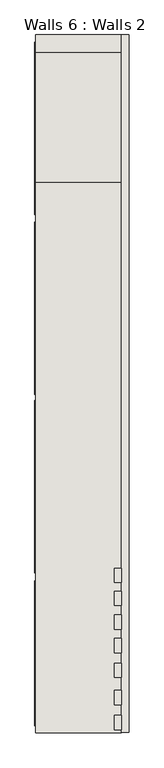
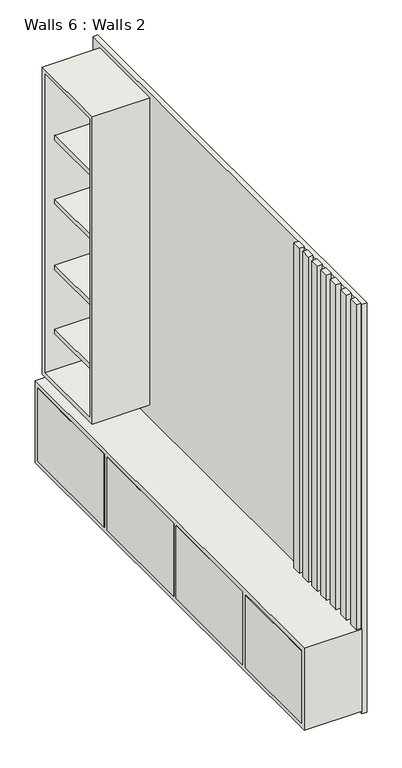
"""IFC4 building model written with IfcOpenShell, lengths in millimetres: wall geometry, Walls 6 : Walls 2."""

from ifc_helpers import new_model, si_unit, frame, origin, place, context, project, spatial, polyline, outline, extrude, faceted_brep, source, transform, mapped, element, save


def walls_6_walls_2_a14d7d6d(model_context):
    return source(origin(), model_context, "Body", "SolidModel", [
        extrude(outline(polyline([(-1167.1478577, -3563.611411), (-1167.1478577, -3052.3039411), (-1164.5681702, -3052.3039411), (-1164.5681702, -3563.611411), (-1167.1478577, -3563.611411)])), frame((0.0, 0.0, 6440.932709), z_axis=(0.0, 0.0, 1.0), x_axis=(1.0, 0.0, 0.0)), (0.0, 0.0, 1.0), 406.4),
        extrude(outline(polyline([(-1167.1478577, -3023.861411), (-1167.1478577, -2414.261411), (-1164.5681702, -2414.261411), (-1164.5681702, -3023.861411), (-1167.1478577, -3023.861411)])), frame((0.0, 0.0, 6440.932709), z_axis=(0.0, 0.0, 1.0), x_axis=(1.0, 0.0, 0.0)), (0.0, 0.0, 1.0), 406.4),
        extrude(outline(polyline([(-1167.1478577, -2393.557676), (-1167.1478577, -1783.957676), (-1164.5681702, -1783.957676), (-1164.5681702, -2393.557676), (-1167.1478577, -2393.557676)])), frame((0.0, 0.0, 6440.932709), z_axis=(0.0, 0.0, 1.0), x_axis=(1.0, 0.0, 0.0)), (0.0, 0.0, 1.0), 406.4),
        extrude(outline(polyline([(-1167.1478577, -1758.557676), (-1167.1478577, -1148.957676), (-1164.5681702, -1148.957676), (-1164.5681702, -1758.557676), (-1167.1478577, -1758.557676)])), frame((0.0, 0.0, 6440.932709), z_axis=(0.0, 0.0, 1.0), x_axis=(1.0, 0.0, 0.0)), (0.0, 0.0, 1.0), 406.4),
        extrude(outline(polyline([(-885.1681702, -3577.3260888), (-885.1681702, -3526.5260888), (-859.7681702, -3526.5260888), (-859.7681702, -3577.3260888), (-885.1681702, -3577.3260888)])), frame((0.0, 0.0, 6872.732709), z_axis=(0.0, 0.0, 1.0), x_axis=(1.0, 0.0, 0.0)), (0.0, 0.0, 1.0), 1815.6625633),
        extrude(outline(polyline([(-885.1681702, -3489.4392633), (-885.1681702, -3438.6392633), (-859.7681702, -3438.6392633), (-859.7681702, -3489.4392633), (-885.1681702, -3489.4392633)])), frame((0.0, 0.0, 6872.732709), z_axis=(0.0, 0.0, 1.0), x_axis=(1.0, 0.0, 0.0)), (0.0, 0.0, 1.0), 1815.6625633),
        extrude(outline(polyline([(-885.1681702, -3222.7392633), (-885.1681702, -3171.9392633), (-859.7681702, -3171.9392633), (-859.7681702, -3222.7392633), (-885.1681702, -3222.7392633)])), frame((0.0, 0.0, 6872.732709), z_axis=(0.0, 0.0, 1.0), x_axis=(1.0, 0.0, 0.0)), (0.0, 0.0, 1.0), 1815.6625633),
        extrude(outline(polyline([(-885.1681702, -3393.1760888), (-885.1681702, -3342.3760888), (-859.7681702, -3342.3760888), (-859.7681702, -3393.1760888), (-885.1681702, -3393.1760888)])), frame((0.0, 0.0, 6872.732709), z_axis=(0.0, 0.0, 1.0), x_axis=(1.0, 0.0, 0.0)), (0.0, 0.0, 1.0), 1815.6625633),
        extrude(outline(polyline([(-885.1681702, -3305.2892633), (-885.1681702, -3254.4892633), (-859.7681702, -3254.4892633), (-859.7681702, -3305.2892633), (-885.1681702, -3305.2892633)])), frame((0.0, 0.0, 6872.732709), z_axis=(0.0, 0.0, 1.0), x_axis=(1.0, 0.0, 0.0)), (0.0, 0.0, 1.0), 1815.6625633),
        extrude(outline(polyline([(-885.1681702, -3139.1760888), (-885.1681702, -3088.3760888), (-859.7681702, -3088.3760888), (-859.7681702, -3139.1760888), (-885.1681702, -3139.1760888)])), frame((0.0, 0.0, 6872.732709), z_axis=(0.0, 0.0, 1.0), x_axis=(1.0, 0.0, 0.0)), (0.0, 0.0, 1.0), 1815.6625633),
        extrude(outline(polyline([(-885.1681702, -3057.9595435), (-885.1681702, -3007.1595435), (-859.7681702, -3007.1595435), (-859.7681702, -3057.9595435), (-885.1681702, -3057.9595435)])), frame((0.0, 0.0, 6872.732709), z_axis=(0.0, 0.0, 1.0), x_axis=(1.0, 0.0, 0.0)), (0.0, 0.0, 1.0), 1815.6625633),
        extrude(outline(polyline([(-1164.5681702, -3587.357676), (-1164.5681702, -1123.557676), (-859.7681702, -1123.557676), (-859.7681702, -3587.357676), (-1164.5681702, -3587.357676)])), frame((0.0, 0.0, 6415.532709), z_axis=(0.0, 0.0, 1.0), x_axis=(1.0, 0.0, 0.0)), (0.0, 0.0, 1.0), 457.2),
        extrude(outline(polyline([(-1113.7681702, -1618.857676), (-1113.7681702, -1212.457676), (-885.1681702, -1212.457676), (-885.1681702, -1618.857676), (-1113.7681702, -1618.857676)])), frame((0.0, 0.0, 8253.2679591), z_axis=(0.0, 0.0, 1.0), x_axis=(1.0, 0.0, 0.0)), (0.0, 0.0, 1.0), 25.4),
        extrude(outline(polyline([(-1113.7681702, -1618.857676), (-1113.7681702, -1212.457676), (-885.1681702, -1212.457676), (-885.1681702, -1618.857676), (-1113.7681702, -1618.857676)])), frame((0.0, 0.0, 7897.6679591), z_axis=(0.0, 0.0, 1.0), x_axis=(1.0, 0.0, 0.0)), (0.0, 0.0, 1.0), 25.4),
        extrude(outline(polyline([(-1113.7681702, -1618.857676), (-1113.7681702, -1212.457676), (-885.1681702, -1212.457676), (-885.1681702, -1618.857676), (-1113.7681702, -1618.857676)])), frame((0.0, 0.0, 7529.3679591), z_axis=(0.0, 0.0, 1.0), x_axis=(1.0, 0.0, 0.0)), (0.0, 0.0, 1.0), 25.4),
        extrude(outline(polyline([(-1113.7681702, -1618.857676), (-1113.7681702, -1212.457676), (-885.1681702, -1212.457676), (-885.1681702, -1618.857676), (-1113.7681702, -1618.857676)])), frame((0.0, 0.0, 7172.3696931), z_axis=(0.0, 0.0, 1.0), x_axis=(1.0, 0.0, 0.0)), (0.0, 0.0, 1.0), 25.4),
        faceted_brep([(-1164.5681702, -1644.257676, 8662.9952722), (-1164.5681702, -1187.057676, 8662.9952722), (-1164.5681702, -1187.057676, 6946.79238), (-1164.5681702, -1644.257676, 6946.79238), (-1164.5681702, -1618.857676, 8637.5952722), (-1164.5681702, -1618.857676, 6972.19238), (-1164.5681702, -1212.457676, 6972.19238), (-1164.5681702, -1212.457676, 8637.5952722), (-859.7681702, -1644.257676, 8662.9952722), (-859.7681702, -1644.257676, 6946.79238), (-859.7681702, -1187.057676, 6946.79238), (-859.7681702, -1187.057676, 8662.9952722), (-885.1681702, -1618.857676, 8637.5952722), (-885.1681702, -1212.457676, 8637.5952722), (-885.1681702, -1212.457676, 6972.19238), (-885.1681702, -1618.857676, 6972.19238)], [[[0, 1, 2, 3], [4, 5, 6, 7]], [[8, 9, 10, 11]], [[1, 0, 8, 11]], [[2, 1, 11, 10]], [[3, 2, 10, 9]], [[0, 3, 9, 8]], [[12, 13, 14, 15]], [[12, 15, 5, 4]], [[15, 14, 6, 5]], [[14, 13, 7, 6]], [[13, 12, 4, 7]]]),
        extrude(outline(polyline([(-859.7681702, -3587.357676), (-859.7681702, -1123.557676), (-834.3681702, -1123.557676), (-834.3681702, -3587.357676), (-859.7681702, -3587.357676)])), frame((0.0, 0.0, 6400.8), z_axis=(0.0, 0.0, 1.0), x_axis=(1.0, 0.0, 0.0)), (0.0, 0.0, 1.0), 2287.5952722),
    ])


if __name__ == "__main__":
    model = new_model("IFC4")
    model_context = context("Model", 3, world=origin())
    ifc_project = project(units=[si_unit("LENGTHUNIT", "METRE", prefix="MILLI")], contexts=[model_context])
    site = spatial("IfcSite", under=ifc_project)
    building = spatial("IfcBuilding", under=site)
    placement = place(None, origin())
    walls_6_walls_2_shape = walls_6_walls_2_a14d7d6d(model_context)
    element("IfcWall", 1, ObjectType="Walls 6 : Walls 2", at=placement, inside=building, context=model_context, shape_type="MappedRepresentation", body=[
        mapped(walls_6_walls_2_shape, transform((0.0, 0.0, 0.0), x_axis=(1.0, 0.0, 0.0), y_axis=(0.0, 1.0, 0.0), z_axis=(0.0, 0.0, 1.0))),
    ])
    save(model, "model.ifc")

# Revit data of these elements
# Element 1 (IfcWall, "Walls 6 : Walls 2")
#   Materials on its faces: "drawers", "metal", "wood"
# Materials
#   "drawers": class "Generic", colour RGB 121 66 39, transparency 0, Cost = 0
#   "metal": class "Generic", colour RGB 76 25 7, transparency 0, Cost = 0
#   "wood": class "Generic", colour RGB 255 226 181, transparency 0, Cost = 0
